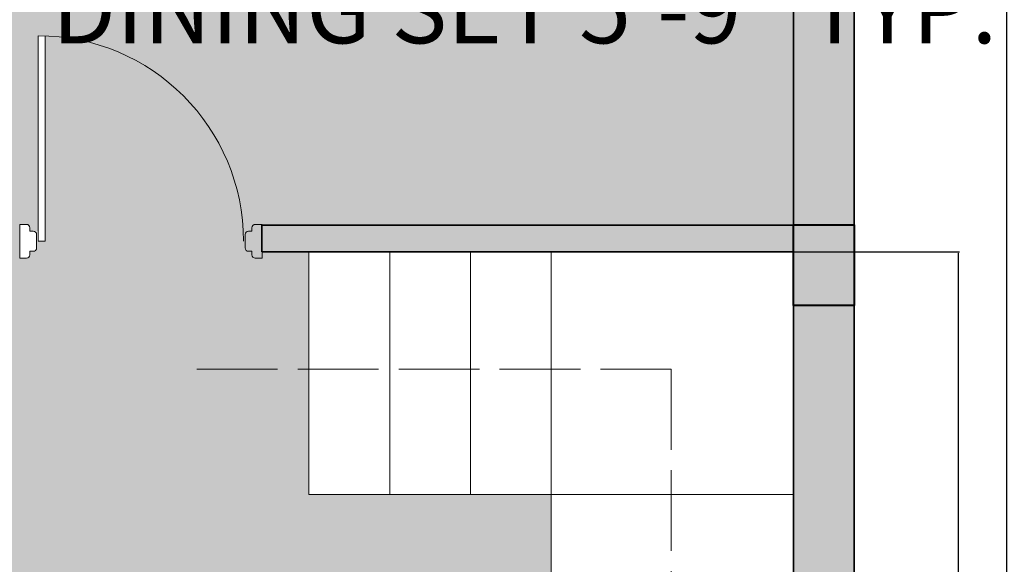
# Model space of a CAD drawing. Units: inches. Extents: x 1077 to 2505, y 1892 to 2728.
# Tile 9 of 26: x 1433 to 1579, y 2257 to 2338. Entities that reach past the tile are written whole.
import ezdxf

# ---------------------------------------------------------------- set-up
doc = ezdxf.new("R2010")
doc.units = ezdxf.units.IN
doc.linetypes.add('ACAD_ISO02W100', pattern=[15, 12, -3])
doc.layers.get('Defpoints').update_dxf_attribs({"color": 220, "linetype": 'ACAD_ISO02W100'})
for name, color, linetype, lineweight in [('00 FURNITURE', 15, 'Continuous', 15), ('A-ANNO-DIMS', 2, 'Continuous', 18), ('A-ANNO-STRS', 220, 'ACAD_ISO02W100', 13), ('A-COLS', 7, 'Continuous', 40), ('A-DOOR', 4, 'Continuous', 18), ('A-FLOR-FIXT', 8, 'Continuous', 13), ('A-FLOR-STRS', 7, 'Continuous', 18), ('A-WALL-PATT', 7, 'Continuous', 9), ('A_TEXT_SMALL', 18, 'Continuous', 13), ('WALL', 7, 'Continuous', 35)]:
    doc.layers.add(name, color=color, linetype=linetype, lineweight=lineweight)
doc.layers.add('A-FLOR-PATT', color=254, linetype='Continuous', lineweight=9, true_color=0xd7ebd2)
doc.styles.get("Standard").update_dxf_attribs({"font": 'arial.ttf'})
doc.dimstyles.get("Standard").update_dxf_attribs({"dimtxt": 10.18, "dimasz": 0.18, "dimexe": 0.18, "dimexo": 0.0625, "dimgap": 0.09, "dimtad": 0, "dimtih": 1, "dimtoh": 1, "dimdec": 0, "dimzin": 0, "dimdsep": 46, "dimlunit": 3, "dimtxsty": 'Standard', "dimcen": 0.09, "dimadec": 0, "dimazin": 0, "dimtfac": 1, "dimtdec": 0, "dimtofl": 0, "dimtmove": 0, "dimatfit": 3, "dimfxl": 1, "dimtolj": 1, "dimtzin": 0, "dimarcsym": 0})

# ---------------------------------------------------------------- blocks, each defined once
blk = doc.blocks.new('DDD')
at = {"layer": '00 FURNITURE'}
for p, q in [((-12579.77, -15859.53), (-12579.77, -15829.05)), ((-12578.77, -15859.53), (-12578.77, -15829.03)), ((-12612.02, -15857.03), (-12612.02, -15862.03)), ((-12611.02, -15857.03), (-12612.02, -15857.03)), ((-12610.52, -15858.03), (-12610.52, -15857.53)), ((-12577.52, -15858.03), (-12577.52, -15857.53)), ((-12577.02, -15857.03), (-12576.02, -15857.03)), ((-12576.02, -15857.03), (-12576.02, -15862.03)), ((-12578.77, -15859.53), (-12579.77, -15859.53)), ((-12612.02, -15862.03), (-12611.02, -15862.03)), ((-12610.52, -15861.53), (-12610.52, -15861.03)), ((-12577.52, -15861.53), (-12577.52, -15861.03)), ((-12576.02, -15862.03), (-12577.02, -15862.03))]:
    blk.add_line(p, q, dxfattribs=at)
for points in [[(-12610.52, -15861.03), (-12610.02, -15861.03, 0.414214), (-12609.52, -15860.53), (-12609.52, -15858.53, 0.414214), (-12610.02, -15858.03), (-12610.52, -15858.03)], [(-12577.52, -15861.03), (-12578.02, -15861.03, -0.414214), (-12578.52, -15860.53), (-12578.52, -15858.53, -0.414214), (-12578.02, -15858.03), (-12577.52, -15858.03)]]:
    blk.add_lwpolyline(points, format="xyb", dxfattribs=at)
for centre, radius, start, end in [((-12578.77, -15859.53), 30.5, 90, 180), ((-12611.02, -15857.53), 0.5, 0, 90), ((-12577.02, -15857.53), 0.5, 90, 180), ((-12611.02, -15861.53), 0.5, 270, 0), ((-12577.02, -15861.53), 0.5, 180, 270)]:
    blk.add_arc(centre, radius, start, end, dxfattribs=at)
blk = doc.blocks.new('reh-flat-2')
at = {"layer": 'A_TEXT_SMALL'}
for p, q in [((486053827.2, -394630231.2), (486054182.4, -394629799.8)), ((486054182.4, -394629799.8), (486054596.6, -394630140.9)), ((486053979.5, -394630126.3), (486054157.1, -394629910.6)), ((486054228.6, -394629903.6), (486054483.5, -394630113.5)), ((486054596.6, -394630140.9), (486054241.4, -394630572.3)), ((486054241.3, -394630407.7), (486053986.4, -394630197.8)), ((486054490.4, -394630185), (486054312.8, -394630400.7)), ((486054241.4, -394630572.3), (486053827.2, -394630231.2))]:
    blk.add_line(p, q, dxfattribs=at)
for centre, radius in [((486054234.9, -394630155.7), 38.1), ((486054004.1, -394630296.2), 20.1), ((486054072.7, -394630352.7), 20.1), ((486054141.4, -394630409.3), 20.1)]:
    blk.add_circle(centre, radius, dxfattribs=at)
for centre, start, end in [((486054196.3, -394629942.9), 50.5305, 140.5305), ((486054018.7, -394630158.5), 140.5305, 230.5305), ((486054451.2, -394630152.8), 320.5305, 50.5305), ((486054273.6, -394630368.4), 230.5305, 320.5305)]:
    blk.add_arc(centre, 50.8, start, end, dxfattribs=at)
blk = doc.blocks.new('C1')
h = blk.add_hatch(color=256)
h.dxf.hatch_style = 1
h.paths.add_polyline_path([(1668.56, 2445.41), (1677.56, 2445.41), (1677.56, 2457.41), (1668.56, 2457.41)])
for p, q in [((1668.56, 2457.41), (1677.56, 2457.41)), ((1668.56, 2445.41), (1668.56, 2457.41)), ((1677.56, 2457.41), (1677.56, 2445.41)), ((1677.56, 2445.41), (1668.56, 2445.41))]:
    blk.add_line(p, q)
blk = doc.blocks.new('*D14')
at = {"layer": 'A-ANNO-DIMS', "color": 0, "lineweight": -2, "transparency": 16777216}
for p, q in [((1555.59, 2651.66), (1579.43, 2651.66)), ((1579.25, 2651.48), (1579.25, 2375.3)), ((1579.25, 2088.54), (1579.25, 2364.72)), ((1555.59, 2088.36), (1579.43, 2088.36))]:
    blk.add_line(p, q, dxfattribs=at)
at = {"layer": 'A-ANNO-DIMS', "color": 0, "transparency": 16777216}
for points in [[(1579.22, 2651.48), (1579.28, 2651.48), (1579.25, 2651.66)], [(1579.22, 2088.54), (1579.28, 2088.54), (1579.25, 2088.36)]]:
    blk.add_solid(points, dxfattribs=at)
at = {"layer": 'Defpoints', "color": 0, "transparency": 16777216}
for p in [(1555.53, 2651.66), (1555.53, 2088.36), (1579.25, 2088.36)]:
    blk.add_point(p, dxfattribs=at)
at = {"layer": 'A-ANNO-DIMS', "color": 0, "transparency": 16777216, "insert": (1579.25, 2370.01), "char_height": 10.18, "attachment_point": 5}
blk.add_mtext('\\A1;46\'-11"', dxfattribs=at)
blk = doc.blocks.new('STAIR-PLAN-RETURN')
for p, q in [((0, 163.08), (0, 127.08)), ((12, 163.08), (12, 127.08)), ((24, 163.08), (24, 127.08)), ((36, 163.08), (36, 0)), ((36, 163.08), (36, 127.08)), ((0, 127.08), (72, 127.08))]:
    blk.add_line(p, q)
blk = doc.blocks.new('STAIR-DIRECTION')
for p, q in [((0, 107.9), (70.51, 107.9)), ((70.51, 107.9), (70.51, 0)), ((70.51, 0.8), (65.28, 12.48)), ((65.28, 12.48), (70.51, 1.21)), ((70.51, 0), (75.75, 12.88)), ((75.75, 12.88), (70.51, 0.8))]:
    blk.add_line(p, q)
blk = doc.blocks.new('*D36')
at = {"layer": 'A-ANNO-DIMS', "color": 0, "lineweight": -2, "transparency": 16777216}
for p, q in [((1365.09, 2349.48), (1365.09, 2339.05)), ((1433.87, 2349.48), (1433.87, 2339.05)), ((1365.27, 2339.23), (1433.69, 2339.23)), ((1433.87, 2339.23), (1434.05, 2339.23))]:
    blk.add_line(p, q, dxfattribs=at)
at = {"layer": 'A-ANNO-DIMS', "color": 0, "transparency": 16777216}
for points in [[(1365.27, 2339.26), (1365.27, 2339.2), (1365.09, 2339.23)], [(1433.69, 2339.26), (1433.69, 2339.2), (1433.87, 2339.23)]]:
    blk.add_solid(points, dxfattribs=at)
at = {"layer": 'Defpoints', "color": 0, "transparency": 16777216}
for p in [(1365.09, 2349.54), (1433.87, 2349.54), (1433.87, 2339.23)]:
    blk.add_point(p, dxfattribs=at)
at = {"layer": 'A-ANNO-DIMS', "color": 0, "transparency": 16777216, "insert": (1507.58, 2339.23), "char_height": 10.18, "attachment_point": 5}
blk.add_mtext('\\A1;DINING SET 5\'-9" TYP.', dxfattribs=at)
blk = doc.blocks.new('*D44')
at = {"layer": 'A-ANNO-DIMS', "color": 0, "lineweight": -2, "transparency": 16777216}
for p, q in [((1547.59, 2303.16), (1572.17, 2303.16)), ((1571.99, 2302.98), (1571.99, 2226.98)), ((1571.99, 2140.26), (1571.99, 2216.26)), ((1547.59, 2140.08), (1572.17, 2140.08))]:
    blk.add_line(p, q, dxfattribs=at)
at = {"layer": 'A-ANNO-DIMS', "color": 0, "transparency": 16777216}
for points in [[(1571.96, 2302.98), (1572.02, 2302.98), (1571.99, 2303.16)], [(1571.96, 2140.26), (1572.02, 2140.26), (1571.99, 2140.08)]]:
    blk.add_solid(points, dxfattribs=at)
at = {"layer": 'Defpoints', "color": 0, "transparency": 16777216}
for p in [(1547.53, 2303.16), (1571.99, 2303.16), (1547.53, 2140.08)]:
    blk.add_point(p, dxfattribs=at)
at = {"layer": 'A-ANNO-DIMS', "color": 0, "transparency": 16777216, "insert": (1571.99, 2221.62), "char_height": 10.18, "attachment_point": 5}
blk.add_mtext('\\A1;RETURN STAIR 13\'-7" TYP.', dxfattribs=at)

msp = doc.modelspace()

# ---------------------------------------------------------------- hatches: boundary and pattern name
at = {"layer": 'A-FLOR-PATT', "transparency": 33554559}
h = msp.add_hatch(color=256, dxfattribs=at)
h.dxf.hatch_style = 1
h.paths.add_polyline_path([(1395.53, 2577.16), (1374.83, 2577.16), (1350.83, 2577.19), (1350.83, 2577.16), (1329.53, 2577.16), (1329.53, 2480.16), (1329.53, 2469.16), (1325.53, 2469.16), (1325.53, 2515.13), (1307.53, 2515.13), (1307.53, 2577.16), (1269.31, 2577.16), (1221.31, 2577.15), (1221.31, 2577.16), (1187.53, 2577.16), (1187.53, 2433.16), (1289.53, 2433.16), (1289.53, 2429.16), (1263.53, 2429.16), (1187.53, 2429.16), (1187.53, 2395.02), (1187.53, 2395.02), (1187.53, 2371.02), (1187.53, 2371.02), (1187.53, 2307.16), (1259.53, 2307.16), (1259.53, 2399.16), (1263.53, 2399.16), (1263.53, 2307.16), (1289.53, 2307.16), (1289.53, 2306.23), (1325.53, 2306.23), (1325.53, 2307.16), (1329.53, 2307.16), (1329.53, 2306.23), (1365.53, 2306.23), (1365.53, 2307.16), (1432.53, 2307.16), (1432.53, 2088.16), (1547.53, 2088.16), (1547.53, 2140.08), (1511.53, 2140.08), (1511.53, 2267.16), (1475.53, 2267.16), (1475.53, 2303.16), (1468.53, 2303.16), (1468.53, 2307.16), (1547.53, 2307.16), (1547.53, 2348.22), (1547.53, 2396.22), (1547.53, 2429.16), (1435.53, 2429.16), (1435.53, 2433.16), (1476.35, 2433.16), (1476.35, 2451.18), (1547.53, 2451.18), (1547.53, 2577.16), (1499.53, 2577.16), (1499.53, 2586.16), (1547.53, 2586.16), (1547.53, 2642.16), (1518.18, 2642.16), (1518.18, 2642.05), (1494.15, 2642.05), (1494.15, 2642.16), (1469.53, 2642.16), (1469.53, 2577.16), (1399.53, 2577.16), (1399.53, 2429.16), (1325.53, 2429.16), (1325.53, 2433.16), (1329.53, 2433.16), (1395.53, 2433.16), (1395.53, 2480.16), (1359.53, 2480.16), (1359.53, 2484.16), (1395.53, 2484.16)])
h.paths.add_polyline_path([(1357.65, 2482.07), (1355.65, 2482.07), (1355.65, 2481.07, 0.414214), (1356.65, 2480.07), (1344.65, 2480.07), (1344.65, 2477.06), (1343.27, 2477.06), (1343.27, 2480.07), (1330.65, 2480.07, -0.414214), (1329.65, 2481.07), (1329.65, 2484.07), (1331.65, 2484.07), (1331.65, 2510.07, -0.446908)], flags=16)
h.paths.add_polyline_path([(1305.09, 2559.18), (1288.89, 2559.18), (1288.89, 2575.38), (1305.09, 2575.38)], flags=16)
h.paths.add_polyline_path([(1304.19, 2560.08), (1289.79, 2560.08), (1289.79, 2574.48), (1304.19, 2574.48)], flags=0)
h.paths.add_polyline_path([(1287.99, 2500.68, -0.414214), (1287.09, 2499.78), (1265.14, 2499.78), (1224.09, 2499.78, -0.414214), (1223.19, 2500.68), (1223.19, 2557.16), (1223.19, 2571.74), (1223.19, 2575.38), (1287.99, 2575.38), (1287.99, 2571.74), (1287.09, 2571.74, -0.414214), (1287.99, 2570.84)], flags=16)
h.paths.add_polyline_path([(1292.98, 2569.05, -1), (1300.92, 2569.05, -1)], flags=0)
h.paths.add_polyline_path([(1293.32, 2569.05, -1), (1300.58, 2569.05, -1)], flags=0)
h.paths.add_polyline_path([(1322.8, 2462.21), (1322.8, 2431.71), (1323.05, 2430.71), (1323.05, 2431.71), (1321.8, 2431.71), (1321.8, 2462.19, 0.404641), (1292.3, 2431.71), (1292.05, 2430.71, -0.414214), (1291.55, 2430.21), (1291.05, 2430.21), (1291.05, 2429.71, -0.414214), (1290.55, 2429.21), (1289.55, 2429.21), (1289.55, 2434.21), (1290.55, 2434.21, -0.414214), (1291.05, 2433.71), (1291.05, 2433.21), (1291.55, 2433.21, -0.414214), (1292.05, 2432.71), (1292.3, 2431.71, -0.414214)], flags=16)
h.paths.add_polyline_path([(1287.82, 2548.28, 0.292232), (1279.17, 2536.8, 0.052719), (1223.93, 2548.28), (1223.28, 2548.28), (1223.28, 2557.16), (1223.93, 2557.16), (1245.42, 2557.16, -0.117785), (1245.77, 2557.93, -0.059418), (1254.87, 2567.02, -0.379859), (1257.28, 2566.88, -0.02509), (1261.41, 2563.32, -0.025935), (1265.65, 2567.02, -0.379859), (1268.06, 2566.88, -0.061767), (1277.52, 2557.43, -0.069393), (1277.82, 2557.16), (1287.82, 2557.16)], flags=0)
h.paths.add_polyline_path([(1263.47, 2548.28), (1260.56, 2548.28, -0.015371), (1258.01, 2546.13, -0.429576), (1255.37, 2546.06, -0.016036), (1252.69, 2548.28), (1223.28, 2548.28), (1223.28, 2554.42), (1246.78, 2554.42, 0.055344), (1255.37, 2546.06, 0.331768), (1257.52, 2545.74, 0.027343), (1262, 2549.64, 0.00919)], flags=0)
h.paths.add_polyline_path([(1295.56, 2568.34), (1296.87, 2569.09), (1296.87, 2570.6, 0.399698), (1295.39, 2569.05, 0.119004)], flags=0)
h.paths.add_polyline_path([(1295.21, 2569.05, -1), (1298.68, 2569.05, -1)], flags=0)
h.paths.add_polyline_path([(1296.95, 2568.96), (1297.03, 2569), (1297.03, 2569.09), (1296.99, 2569.11), (1296.91, 2568.98)], flags=0)
h.paths.add_polyline_path([(1402.28, 2462.19, -0.414214), (1432.78, 2431.69), (1433.03, 2432.69), (1432.78, 2431.69, 0.404641), (1403.28, 2462.17), (1403.28, 2431.69), (1402.03, 2431.69), (1402.03, 2430.69, -0.414214), (1401.53, 2430.19), (1401.03, 2430.19), (1401.03, 2429.69, -0.414214), (1400.53, 2429.19), (1399.53, 2429.19), (1399.53, 2434.19), (1400.53, 2434.19, -0.414214), (1401.03, 2433.69), (1401.03, 2433.19), (1401.53, 2433.19, -0.414214), (1402.03, 2432.69)], flags=16)
h.paths.add_polyline_path([(1470.16, 2535.21, -0.414214), (1471.06, 2536.11), (1527.54, 2536.11), (1542.12, 2536.11), (1545.76, 2536.11), (1545.76, 2471.31), (1542.12, 2471.31), (1542.12, 2472.21, -0.414214), (1541.22, 2471.31), (1471.06, 2471.31, -0.414214), (1470.16, 2472.21), (1470.16, 2494.16)], flags=16)
h.paths.add_polyline_path([(1483.07, 2536.11, 0.253465), (1480.11, 2526.15, 0.2538), (1470.15, 2523.19)], flags=16)
h.paths.add_polyline_path([(1223.19, 2512.69, 0.253465), (1233.14, 2509.74, 0.2538), (1236.1, 2499.77)], flags=16)
h.paths.add_polyline_path([(1469.77, 2578.72), (1469.77, 2581.72), (1471.77, 2581.72), (1471.77, 2607.72, -0.01951), (1473.77, 2607.68), (1473.77, 2579.72), (1473.77, 2578.72, -0.414214), (1472.77, 2577.72), (1470.77, 2577.72, -0.414214)], flags=16)
h.paths.add_polyline_path([(1382.46, 2398.13), (1395.04, 2398.13), (1395.04, 2399.74), (1382.46, 2399.74)], flags=16)
h.paths.add_polyline_path([(1379.94, 2397.18), (1379.94, 2389.82), (1380.5, 2389.82), (1380.5, 2396.05, -0.41429), (1381.06, 2396.61), (1396.47, 2396.61, -0.414213), (1397.03, 2396.05), (1397.03, 2389.82), (1397.59, 2389.82), (1397.59, 2397.18)], flags=16)
h.paths.add_polyline_path([(1263.37, 2428.14), (1263.37, 2426.14, -0.414214), (1262.37, 2425.14), (1261.37, 2425.14), (1233.41, 2425.14, 0.400854), (1259.37, 2401.04), (1259.37, 2401.14), (1261.37, 2401.14, -0.446908), (1233.37, 2427.14), (1259.37, 2427.14), (1259.37, 2429.14), (1262.37, 2429.14, -0.414214)], flags=16)
h.paths.add_polyline_path([(1404.79, 2398.13), (1417.37, 2398.13), (1417.37, 2399.74), (1404.79, 2399.74)], flags=16)
h.paths.add_polyline_path([(1402.27, 2397.18), (1404.79, 2398.13), (1417.37, 2398.13), (1419.92, 2397.18)], flags=16)
h.paths.add_polyline_path([(1432.26, 2383.16), (1432.26, 2370.59), (1433.87, 2370.59), (1433.87, 2383.16)], flags=16)
h.paths.add_polyline_path([(1431.3, 2385.69), (1423.84, 2385.69), (1423.84, 2385.13), (1430.18, 2385.13, -0.41429), (1430.74, 2384.57), (1430.74, 2369.16, -0.414237), (1430.18, 2368.6), (1423.84, 2368.6), (1423.84, 2368.03), (1431.3, 2368.03)], flags=16)
h.paths.add_polyline_path([(1417.37, 2351.16), (1417.37, 2349.54), (1418.9, 2349.54, 0.414236), (1419.92, 2350.56), (1419.92, 2352.11)], flags=16)
h.paths.add_polyline_path([(1395.04, 2351.16), (1395.04, 2349.54), (1396.58, 2349.54, 0.414235), (1397.59, 2350.56), (1397.59, 2352.11)], flags=16)
h.paths.add_polyline_path([(1366.7, 2370.05), (1365.09, 2370.05), (1365.09, 2368.52, 0.414235), (1366.11, 2367.5), (1367.66, 2367.5)], flags=16)
h.paths.add_polyline_path([(1419.36, 2359.47), (1419.36, 2353.24, -0.41419), (1418.8, 2352.68), (1403.39, 2352.68, -0.414137), (1402.83, 2353.24), (1402.83, 2359.47), (1397.03, 2359.47), (1397.03, 2353.24, -0.414189), (1396.47, 2352.68), (1381.06, 2352.68, -0.414137), (1380.5, 2353.24), (1380.5, 2359.47)], flags=16)
h.paths.add_polyline_path([(1222.29, 2559.18), (1206.09, 2559.18), (1206.09, 2575.38), (1222.29, 2575.38)], flags=16)
h.paths.add_polyline_path([(1221.39, 2560.08), (1206.99, 2560.08), (1206.99, 2574.48), (1221.39, 2574.48)], flags=0)
h.paths.add_polyline_path([(1482, 2577.72), (1482, 2580.73), (1483.38, 2580.73), (1483.38, 2577.72), (1484.77, 2577.72), (1484.77, 2574.72), (1483.38, 2574.72), (1483.38, 2577.72)], flags=16)
h.paths.add_polyline_path([(1266.37, 2415.53), (1266.37, 2414.14), (1263.37, 2414.14), (1263.37, 2415.53), (1260.36, 2415.53), (1260.36, 2416.91), (1263.37, 2416.91), (1263.37, 2415.53)], flags=16)
h.paths.add_polyline_path([(1210.26, 2569.05, -1), (1218.19, 2569.05, -1)], flags=0)
h.paths.add_polyline_path([(1210.6, 2569.05, -1), (1217.85, 2569.05, -1)], flags=0)
h.paths.add_polyline_path([(1212.84, 2568.34), (1214.15, 2569.09), (1214.15, 2570.6, 0.399698), (1212.67, 2569.05, 0.119004)], flags=0)
h.paths.add_polyline_path([(1212.49, 2569.05, -1), (1215.96, 2569.05, -1)], flags=0)
h.paths.add_polyline_path([(1214.23, 2568.96), (1214.3, 2568.91), (1214.3, 2569)], flags=0)
h.paths.add_polyline_path([(1507.18, 2480.12, 0.052719), (1518.66, 2535.36), (1518.66, 2536.01), (1527.54, 2536.01), (1527.54, 2535.36), (1527.54, 2513.88, -0.117785), (1528.31, 2513.53, -0.059418), (1537.4, 2504.43, -0.379859), (1537.26, 2502.01, -0.02509), (1533.7, 2497.89, -0.025935), (1537.4, 2493.64, -0.379859), (1537.26, 2491.23, -0.061767), (1527.8, 2481.77, -0.069393), (1527.54, 2481.47), (1527.54, 2471.47), (1518.66, 2471.47, 0.292232)], flags=0)
h.paths.add_polyline_path([(1516.43, 2503.92, -0.016036), (1518.66, 2506.6), (1518.66, 2536.01), (1524.8, 2536.01), (1524.8, 2512.51, 0.055344), (1516.43, 2503.92, 0.331768), (1516.12, 2501.77, 0.027343), (1520.01, 2497.29, 0.00919), (1518.66, 2495.82), (1518.66, 2498.73, -0.015371), (1516.5, 2501.28, -0.429576)], flags=0)
h.paths.add_polyline_path([(1499.63, 2625.5, -0.171636), (1502.82, 2631.01), (1502.82, 2633.37), (1498.68, 2633.37, -0.414214), (1497.7, 2634.36), (1497.7, 2640.66, -0.414214), (1498.68, 2641.64), (1514.82, 2641.64, -0.414214), (1515.81, 2640.66), (1515.81, 2634.36, -0.414214), (1514.82, 2633.37), (1510.69, 2633.37), (1510.69, 2631.01, -0.171636), (1513.88, 2625.5, -0.258205), (1509.31, 2614.47), (1504.19, 2614.47, -0.258205)], flags=16)
h.paths.add_polyline_path([(1501.2, 2625.5, -0.171636), (1504.39, 2631.01), (1509.12, 2631.01, -0.171636), (1512.3, 2625.5, -0.210384), (1509.35, 2616.02), (1504.16, 2616.02, -0.210384)], flags=0)
h.paths.add_polyline_path([(1529.56, 2537.01), (1529.56, 2553.21), (1545.76, 2553.21), (1545.76, 2537.01)], flags=16)
h.paths.add_polyline_path([(1530.46, 2537.91), (1530.46, 2552.31), (1544.86, 2552.31), (1544.86, 2537.91)], flags=0)
h.paths.add_polyline_path([(1535.45, 2545.07, -1), (1543.39, 2545.07, -1)], flags=0)
h.paths.add_polyline_path([(1535.8, 2545.07, -1), (1543.05, 2545.07, -1)], flags=0)
h.paths.add_polyline_path([(1529.56, 2470.41), (1545.76, 2470.41), (1545.76, 2454.21), (1529.56, 2454.21)], flags=16)
h.paths.add_polyline_path([(1541.16, 2544.99), (1540.98, 2544.99, -0.544606), (1538.71, 2543.68), (1538.62, 2543.53, 0.547962)], flags=0)
h.paths.add_polyline_path([(1530.46, 2469.51), (1544.86, 2469.51), (1544.86, 2455.11), (1530.46, 2455.11)], flags=0)
h.paths.add_polyline_path([(1539.47, 2545.14), (1539.42, 2545.22), (1539.38, 2545.14)], flags=0)
h.paths.add_polyline_path([(1543.39, 2462.34, -1), (1535.45, 2462.34, -1)], flags=0)
h.paths.add_polyline_path([(1543.05, 2462.34, -1), (1535.8, 2462.34, -1)], flags=0)
h.paths.add_polyline_path([(1541.16, 2462.27), (1540.98, 2462.27, -0.544606), (1538.71, 2460.96), (1538.62, 2460.8, 0.547962)], flags=0)
h.paths.add_polyline_path([(1539.47, 2462.42), (1539.42, 2462.5), (1539.38, 2462.42)], flags=0)
h.paths.add_polyline_path([(1435.32, 2335.25, -0.414214), (1465.82, 2304.75), (1466.07, 2305.75), (1465.82, 2304.75, 0.404641), (1436.32, 2335.23), (1436.32, 2304.75), (1435.07, 2304.75), (1435.07, 2303.75, -0.414214), (1434.57, 2303.25), (1434.07, 2303.25), (1434.07, 2302.75, -0.414214), (1433.57, 2302.25), (1432.57, 2302.25), (1432.57, 2307.25), (1433.57, 2307.25, -0.414214), (1434.07, 2306.75), (1434.07, 2306.25), (1434.57, 2306.25, -0.414214), (1435.07, 2305.75)], flags=16)
h.paths.add_polyline_path([(1532.13, 2635.71), (1535.43, 2635.71), (1535.43, 2635.89), (1532.13, 2635.89)], flags=16)
edge = h.paths.add_edge_path(flags=16)
edge.add_arc((1535.98, 2632.67), 0.183, 270, 360)
edge.add_line((1536.17, 2632.67), (1536.17, 2639.82))
edge.add_line((1536.17, 2639.82), (1538.29, 2639.82))
edge.add_line((1538.29, 2639.82), (1538.29, 2641.82))
edge.add_line((1538.29, 2641.82), (1533.25, 2641.82))
edge.add_line((1533.25, 2641.82), (1533.25, 2639.82))
edge.add_line((1533.25, 2639.82), (1534.87, 2639.82))
edge.add_line((1534.87, 2639.82), (1534.87, 2639))
edge.add_line((1534.87, 2639), (1533.7, 2639))
edge.add_line((1533.7, 2639), (1533.7, 2639.82))
edge.add_line((1533.7, 2639.82), (1533.25, 2639.82))
edge.add_line((1533.25, 2639.82), (1533.25, 2641.82))
edge.add_line((1533.25, 2641.82), (1538.29, 2641.82))
edge.add_line((1538.29, 2641.82), (1538.29, 2641.34))
edge.add_line((1538.29, 2641.34), (1540.64, 2641.58))
edge.add_line((1540.64, 2641.58), (1540.64, 2641.82))
edge.add_line((1540.64, 2641.82), (1541.5, 2641.82))
edge.add_line((1541.5, 2641.82), (1541.5, 2641.25))
edge.add_line((1541.5, 2641.25), (1541.31, 2639.79))
edge.add_ellipse((1541.09, 2638.95), major_axis=(-1.08, 0), ratio=0.790849, start_angle=180, end_angle=255.2976, ccw=False)
edge.add_line((1542.17, 2638.95), (1542.17, 2638.38))
edge.add_ellipse((1541.09, 2638.38), major_axis=(-1.08, 0), ratio=0.790849, start_angle=0, end_angle=180, ccw=False)
edge.add_line((1540, 2638.38), (1540.01, 2638.87))
edge.add_ellipse((1541.09, 2638.95), major_axis=(-1.08, 0), ratio=0.790849, start_angle=284.7024, end_angle=364.0401, ccw=False)
edge.add_line((1540.78, 2639.75), (1540.78, 2641.25))
edge.add_line((1540.78, 2641.25), (1540.64, 2641.25))
edge.add_line((1540.64, 2641.25), (1538.29, 2641.01))
edge.add_line((1538.29, 2641.01), (1538.29, 2639.82))
edge.add_line((1538.29, 2639.82), (1536.17, 2639.82))
edge.add_line((1536.17, 2639.82), (1536.17, 2632.48))
edge.add_line((1536.17, 2632.48), (1535.98, 2632.48))
h.paths.add_polyline_path([(1496.32, 2250.34, -0.292371), (1498.9, 2247.83, -0.085148), (1501.21, 2208.85, -0.01331), (1500.27, 2098.5, -0.379287), (1497.22, 2095.28, -0.0502), (1441.54, 2095.28, -0.379287), (1438.5, 2098.5, -0.01331), (1437.56, 2208.85, -0.086132), (1439.96, 2248.26, -0.295116), (1442.59, 2250.78, -0.114238)], flags=16)
h.paths.add_polyline_path([(1495.16, 2205.84, -0.355389), (1496.7, 2202.1), (1492.94, 2189.65, -0.398275), (1489.12, 2187.47, 0.113332), (1449.64, 2187.47, -0.398275), (1445.82, 2189.65), (1442.06, 2202.1, -0.355394), (1443.6, 2205.84, -0.265725)], flags=0)
h.paths.add_polyline_path([(1440.37, 2195.72), (1445.94, 2181.67), (1445.94, 2160.63), (1440.84, 2157.26)], flags=0)
h.paths.add_polyline_path([(1498.46, 2195.72), (1497.99, 2157.26), (1492.88, 2160.63), (1492.88, 2181.67)], flags=0)
h.paths.add_polyline_path([(1445.94, 2158.37), (1445.94, 2137.12), (1441.12, 2122.56), (1440.87, 2155.03)], flags=0)
h.paths.add_polyline_path([(1492.88, 2158.37), (1497.96, 2155.03), (1497.71, 2122.56), (1492.88, 2137.12)], flags=0)
h.paths.add_polyline_path([(1489.88, 2130.4), (1494.39, 2107.67, -0.090102), (1444.44, 2107.65), (1448.95, 2130.39, 0.036636)], flags=0)
h.paths.add_polyline_path([(1447.54, 2159.34), (1497.44, 2159.34), (1497.44, 2177.89), (1447.54, 2177.89)], flags=8)
h.paths.add_polyline_path([(1196.44, 2354.84), (1246.65, 2354.84), (1246.65, 2388.43), (1196.44, 2388.43)], flags=24)
h.paths.add_polyline_path([(1296.09, 2360.25), (1353.81, 2360.25), (1353.81, 2393.84), (1296.09, 2393.84)], flags=24)
h.paths.add_polyline_path([(1400.72, 2471.85), (1470.63, 2471.85), (1470.63, 2505.44), (1400.72, 2505.44)], flags=24)
h.paths.add_polyline_path([(1324.78, 2448.48), (1394.95, 2448.48), (1394.95, 2467.02), (1324.78, 2467.02)], flags=24)
h.paths.add_polyline_path([(1335.08, 2531.43), (1389.67, 2531.43), (1389.67, 2565.02), (1335.08, 2565.02)], flags=24)
h.paths.add_polyline_path([(1225.76, 2460), (1295.67, 2460), (1295.67, 2493.58), (1225.76, 2493.58)], flags=24)
h = msp.add_hatch(color=256, dxfattribs=at)
h.dxf.hatch_style = 1
h.paths.add_polyline_path([(1547.53, 2348.22), (1547.53, 2396.22), (1547.53, 2425.11), (1547.53, 2425.11), (1547.53, 2429.16), (1435.53, 2429.16), (1434.03, 2429.21), (1434.03, 2430.19), (1433.03, 2430.19), (1432.78, 2431.69, 0.404641), (1403.28, 2462.17), (1403.28, 2431.69), (1402.03, 2431.69), (1402.03, 2430.19), (1401.03, 2430.19), (1401.03, 2429.19), (1399.53, 2429.19), (1399.53, 2429.19), (1399.53, 2429.16), (1334.67, 2429.16), (1334.67, 2423.95), (1325.67, 2423.95), (1325.67, 2429.16), (1325.53, 2429.16), (1324.05, 2429.24), (1324.05, 2430.21), (1323.05, 2430.21), (1323.05, 2431.71), (1321.8, 2431.71), (1321.8, 2462.19, 0.416544), (1292.05, 2430.73, -0.423614), (1291.55, 2430.21), (1291.05, 2430.21), (1291.05, 2429.21), (1289.55, 2429.21), (1289.53, 2429.21), (1289.53, 2429.16), (1263.37, 2429.16), (1263.37, 2415.53), (1266.37, 2415.53), (1266.37, 2414.14), (1263.37, 2414.14), (1263.37, 2399.16), (1263.53, 2399.16), (1263.53, 2307.16), (1289.53, 2307.16), (1289.53, 2306.23), (1323.26, 2306.23), (1323.26, 2307.21), (1332.26, 2307.21), (1365.53, 2306.23), (1365.53, 2307.16), (1432.53, 2307.16), (1432.57, 2307.16), (1432.57, 2307.25), (1434.07, 2307.25), (1434.07, 2306.25), (1435.32, 2306.25), (1435.32, 2335.25, -0.407346), (1466.07, 2305.73, -0.423614), (1466.57, 2306.25), (1467.07, 2306.25), (1467.07, 2307.25), (1468.57, 2307.25), (1547.53, 2307.16), (1547.53, 2307.2)])
h.paths.add_polyline_path([(1430.74, 2369.16), (1430.74, 2384.57, 0.41429), (1430.18, 2385.13), (1423.84, 2385.13), (1423.84, 2368.6), (1430.18, 2368.6, 0.414237)], flags=16)
h.paths.add_polyline_path([(1432.26, 2383.16), (1432.26, 2370.59), (1433.87, 2370.59), (1433.87, 2383.16)], flags=16)
h.paths.add_polyline_path([(1431.3, 2368.03), (1431.3, 2385.69), (1432.26, 2383.16), (1432.26, 2370.59)], flags=16)
h.paths.add_polyline_path([(1417.37, 2351.16), (1417.37, 2349.54), (1418.9, 2349.54, 0.414236), (1419.92, 2350.56), (1419.92, 2352.11)], flags=16)
h.paths.add_polyline_path([(1403.39, 2352.68), (1418.78, 2352.68, 0.42427), (1419.36, 2353.24), (1419.36, 2359.47), (1402.83, 2359.47), (1402.83, 2353.24, 0.414137)], flags=16)
h.paths.add_polyline_path([(1366.7, 2370.05), (1365.09, 2370.05), (1365.09, 2368.52, 0.414235), (1366.11, 2367.5), (1367.66, 2367.5)], flags=16)
h.paths.add_polyline_path([(1382.46, 2398.13), (1395.04, 2398.13), (1395.04, 2399.74), (1382.46, 2399.74)], flags=16)
h.paths.add_polyline_path([(1396.47, 2396.61), (1381.06, 2396.61, 0.41429), (1380.5, 2396.05), (1380.5, 2389.82), (1397.03, 2389.82), (1397.03, 2396.05, 0.414213)], flags=16)
h.paths.add_polyline_path([(1402.27, 2397.18), (1402.83, 2396.05, -0.414213), (1403.39, 2396.61)], flags=16)
h.paths.add_polyline_path([(1418.8, 2396.61), (1419.36, 2396.61), (1419.36, 2396.05, 0.414237)], flags=16)
h.paths.add_polyline_path([(1404.79, 2398.13), (1417.37, 2398.13), (1417.37, 2399.74), (1404.79, 2399.74)], flags=16)
h.paths.add_polyline_path([(1381.06, 2352.68, -0.414213), (1380.5, 2353.24), (1380.27, 2352.11)], flags=16)
h.paths.add_polyline_path([(1396.58, 2349.54), (1396.58, 2349.54), (1395.04, 2349.54), (1395.04, 2349.54), (1382.46, 2349.54), (1382.46, 2351.16), (1395.04, 2351.16), (1397.59, 2352.11), (1397.59, 2350.56, -0.414235)], flags=16)
h.paths.add_polyline_path([(1379.94, 2397.18), (1382.46, 2398.13), (1395.04, 2398.13), (1397.59, 2397.18)], flags=16)
h.paths.add_polyline_path([(1368.78, 2384.59, 0.414213), (1368.22, 2384.03), (1367.66, 2367.5), (1367.66, 2385.15)], flags=16)
h.paths.add_polyline_path([(1547.53, 2574.38), (1547.51, 2574.38), (1547.51, 2577.16), (1499.53, 2577.16), (1484.77, 2577.44), (1484.77, 2574.72), (1483.38, 2574.72), (1483.38, 2577.72), (1482, 2577.72), (1469.53, 2577.72), (1469.53, 2577.16), (1401.95, 2577.16), (1401.95, 2574.12), (1399.53, 2574.12), (1399.53, 2434.19), (1401.03, 2434.19), (1401.03, 2433.19), (1402.28, 2433.19), (1402.28, 2462.19, -0.407346), (1433.03, 2432.67, -0.423614), (1433.53, 2433.19), (1434.03, 2433.19), (1434.03, 2434.19), (1435.53, 2434.19), (1476.35, 2433.81), (1476.35, 2451.18), (1547.53, 2451.18)])
h.paths.add_polyline_path([(1470.16, 2535.21, -0.414214), (1471.06, 2536.11), (1527.54, 2536.11), (1542.12, 2536.11), (1545.76, 2536.11), (1545.76, 2471.31), (1542.12, 2471.31), (1542.12, 2472.21, -0.414214), (1541.22, 2471.31), (1471.06, 2471.31, -0.414214), (1470.16, 2472.21), (1470.16, 2494.16)], flags=16)
h.paths.add_polyline_path([(1483.07, 2536.11, 0.253465), (1480.11, 2526.15, 0.2538), (1470.15, 2523.19)], flags=16)
h.paths.add_polyline_path([(1525.55, 2481.52, -0.000893), (1524.8, 2482.24), (1524.8, 2471.47), (1527.54, 2471.47), (1527.54, 2472.12), (1527.54, 2481.47, -0.388819)], flags=0)
h.paths.add_polyline_path([(1518.66, 2536.01), (1527.54, 2536.01), (1527.54, 2535.36), (1527.54, 2513.88, -0.117785), (1528.31, 2513.53, -0.059418), (1537.4, 2504.43, -0.379859), (1537.26, 2502.01, -0.02509), (1533.7, 2497.89, 0.033431), (1528.3, 2502.74, 0.308459), (1526.25, 2502.88, 0.047827), (1518.66, 2495.82), (1518.66, 2498.73, -0.015371), (1516.5, 2501.28, -0.429576), (1516.43, 2503.92, -0.016036), (1518.66, 2506.6)], flags=0)
h.paths.add_polyline_path([(1529.56, 2537.01), (1529.56, 2553.21), (1545.76, 2553.21), (1545.76, 2537.01)], flags=16)
h.paths.add_polyline_path([(1530.46, 2537.91), (1530.46, 2552.31), (1544.86, 2552.31), (1544.86, 2537.91)], flags=0)
h.paths.add_polyline_path([(1535.8, 2545.07, -1), (1543.05, 2545.07, -1)], flags=0)
h.paths.add_polyline_path([(1541.16, 2544.99), (1540.98, 2544.99, -0.544606), (1538.71, 2543.68), (1538.62, 2543.53, 0.547962)], flags=0)
h.paths.add_polyline_path([(1539.47, 2545.14), (1539.42, 2545.22), (1539.38, 2545.14)], flags=0)
h.paths.add_polyline_path([(1529.56, 2470.41), (1545.76, 2470.41), (1545.76, 2454.21), (1529.56, 2454.21)], flags=16)
h.paths.add_polyline_path([(1530.46, 2469.51), (1544.86, 2469.51), (1544.86, 2455.11), (1530.46, 2455.11)], flags=0)
h.paths.add_polyline_path([(1535.8, 2462.34, -1), (1543.05, 2462.34, -1)], flags=0)
h.paths.add_polyline_path([(1541.16, 2462.27), (1540.98, 2462.27, -0.544606), (1538.71, 2460.96), (1538.62, 2460.8, 0.547962)], flags=0)
h.paths.add_polyline_path([(1539.47, 2462.42), (1539.42, 2462.5), (1539.38, 2462.42)], flags=0)
h.paths.add_polyline_path([(1395.53, 2574.12), (1392.95, 2574.12), (1392.95, 2577.16), (1374.83, 2577.16), (1350.83, 2577.19), (1350.83, 2577.16), (1332.07, 2577.16), (1332.07, 2574), (1329.53, 2574), (1329.53, 2484.07), (1331.65, 2484.07), (1331.65, 2510.07, -0.423677), (1357.76, 2484.07), (1359.53, 2484.07), (1359.53, 2484.16), (1395.53, 2484.16)], flags=17)
h.paths.add_polyline_path([(1395.53, 2480.16), (1359.06, 2480.16, 0.437533), (1359.53, 2481.55), (1359.53, 2484.16), (1395.53, 2484.16), (1395.53, 2574.12), (1392.95, 2574.12), (1392.95, 2577.16), (1374.83, 2577.16), (1350.83, 2577.19), (1350.83, 2577.16), (1332.07, 2577.16), (1332.07, 2574), (1329.53, 2574), (1329.53, 2484.07), (1329.65, 2484.07), (1329.65, 2481.07), (1329.53, 2480.16), (1329.53, 2469.16), (1325.53, 2469.16), (1325.53, 2515.13), (1307.53, 2515.13), (1307.53, 2577.16), (1269.31, 2577.16), (1221.31, 2577.15), (1221.31, 2577.16), (1187.61, 2577.16), (1187.61, 2574.03), (1187.53, 2433.16), (1289.55, 2433.16), (1289.55, 2434.21), (1291.05, 2434.21), (1291.05, 2433.21), (1292.05, 2433.21), (1292.3, 2431.71, -0.414214), (1322.8, 2462.21), (1323.05, 2432.71, -0.414214), (1323.55, 2433.21), (1324.05, 2433.21), (1324.05, 2434.21), (1325.67, 2434.21), (1325.67, 2435.95), (1334.67, 2435.95), (1334.67, 2433.16), (1395.53, 2433.16)])
h.paths.add_polyline_path([(1344.65, 2480.07), (1344.65, 2477.06), (1343.27, 2477.06), (1343.27, 2480.07), (1332.65, 2480.07, 0.414214), (1333.65, 2481.07), (1333.65, 2482.07), (1331.65, 2482.07), (1331.65, 2484.07), (1331.65, 2510.07, -0.446908), (1357.65, 2482.07), (1355.65, 2482.07), (1355.65, 2481.07, 0.414214), (1356.65, 2480.07)], flags=16)
h.paths.add_polyline_path([(1287.99, 2500.68, -0.414214), (1287.09, 2499.78), (1265.14, 2499.78), (1224.09, 2499.78, -0.414214), (1223.19, 2500.68), (1223.19, 2557.16), (1223.19, 2571.74), (1223.19, 2575.38), (1287.99, 2575.38), (1287.99, 2571.74), (1287.09, 2571.74, -0.414214), (1287.99, 2570.84)], flags=16)
h.paths.add_polyline_path([(1277.77, 2555.17, -0.000893), (1277.05, 2554.42), (1287.82, 2554.42), (1287.82, 2557.16), (1287.17, 2557.16), (1277.82, 2557.16, -0.388819)], flags=0)
h.paths.add_polyline_path([(1223.28, 2548.28), (1223.28, 2557.16), (1223.93, 2557.16), (1245.42, 2557.16, -0.117785), (1245.77, 2557.93, -0.059418), (1254.87, 2567.02, -0.379859), (1257.28, 2566.88, -0.02509), (1261.41, 2563.32, 0.033431), (1256.55, 2557.93, 0.308459), (1256.41, 2555.88, 0.047827), (1263.47, 2548.28), (1260.56, 2548.28, -0.015371), (1258.01, 2546.13, -0.429576), (1255.37, 2546.06, -0.016036), (1252.69, 2548.28)], flags=0)
h.paths.add_polyline_path([(1305.09, 2559.18), (1288.89, 2559.18), (1288.89, 2575.38), (1305.09, 2575.38)], flags=16)
h.paths.add_polyline_path([(1304.19, 2560.08), (1289.79, 2560.08), (1289.79, 2574.48), (1304.19, 2574.48)], flags=0)
h.paths.add_polyline_path([(1300.58, 2569.05, -1), (1293.32, 2569.05, -1)], flags=0)
h.paths.add_polyline_path([(1223.19, 2512.69, 0.253465), (1233.14, 2509.74, 0.2538), (1236.1, 2499.77)], flags=16)
h.paths.add_polyline_path([(1295.56, 2568.34), (1296.87, 2569.09), (1296.87, 2570.6, 0.399698), (1295.39, 2569.05, 0.119004)], flags=0)
h.paths.add_polyline_path([(1295.21, 2569.05, -1), (1298.68, 2569.05, -1)], flags=0)
h.paths.add_polyline_path([(1296.95, 2568.96), (1297.03, 2569), (1297.03, 2569.09), (1296.99, 2569.11), (1296.91, 2568.98)], flags=0)
h.paths.add_polyline_path([(1222.29, 2559.18), (1206.09, 2559.18), (1206.09, 2575.38), (1222.29, 2575.38)], flags=16)
h.paths.add_polyline_path([(1221.39, 2560.08), (1206.99, 2560.08), (1206.99, 2574.48), (1221.39, 2574.48)], flags=0)
h.paths.add_polyline_path([(1217.85, 2569.05, -1), (1210.6, 2569.05, -1)], flags=0)
h.paths.add_polyline_path([(1212.84, 2568.34), (1214.15, 2569.09), (1214.15, 2570.6, 0.399698), (1212.67, 2569.05, 0.119004)], flags=0)
h.paths.add_polyline_path([(1212.49, 2569.05, -1), (1215.96, 2569.05, -1)], flags=0)
h.paths.add_polyline_path([(1214.23, 2568.96), (1214.3, 2569), (1214.3, 2569.09), (1214.26, 2569.11), (1214.19, 2568.98)], flags=0)
h.paths.add_polyline_path([(1259.53, 2399.14), (1259.37, 2399.14), (1259.37, 2401.04, -0.423677), (1233.37, 2427.14), (1259.37, 2427.14), (1259.37, 2429.16), (1187.53, 2429.16), (1187.53, 2395.02), (1187.53, 2395.02), (1187.53, 2371.02), (1187.53, 2371.02), (1187.53, 2311.49), (1187.55, 2311.49), (1187.55, 2307.16), (1259.53, 2307.16)])
h.paths.add_polyline_path([(1323.26, 2295.21), (1323.26, 2304.23), (1289.53, 2304.23), (1289.53, 2303.16), (1187.55, 2303.16), (1187.55, 2299.49), (1178.53, 2299.49), (1178.53, 2267.66), (1178.53, 2219.66), (1182.03, 2219.66), (1182.03, 2267.67), (1184.03, 2267.67), (1184.03, 2219.66), (1187.53, 2219.66), (1187.53, 2153.16), (1228.13, 2153.16), (1276.13, 2153.16), (1276.13, 2153.16), (1324.54, 2153.16), (1324.54, 2154.67), (1325.54, 2154.67), (1325.54, 2155.92), (1296.54, 2155.92, -0.407346), (1326.06, 2186.67, -0.423614), (1325.54, 2187.17), (1325.54, 2187.67), (1324.54, 2187.67), (1324.54, 2189.17), (1325.43, 2295.21)])
h.paths.add_polyline_path([(1432.53, 2307.16), (1365.53, 2307.16), (1365.53, 2306.23), (1365.53, 2303.16), (1428.53, 2303.16), (1428.53, 2221.2), (1428.57, 2221.2), (1428.57, 2197.2), (1428.53, 2197.16), (1428.53, 2303.01), (1404.46, 2303.01), (1404.46, 2221.2), (1329.53, 2221.2), (1329.53, 2307.16), (1325.53, 2307.16), (1325.53, 2295.21), (1325.43, 2295.21), (1324.54, 2189.17), (1324.54, 2187.67), (1326.04, 2187.67, 1.016365), (1326.06, 2186.67, 0.407348), (1296.54, 2155.92), (1325.54, 2155.92), (1325.54, 2154.67), (1324.54, 2154.67), (1324.54, 2153.16), (1329.53, 2153.16), (1329.53, 2144.16), (1432.53, 2144.16)])
h.paths.add_polyline_path([(1361.95, 2194.26), (1361.95, 2193.16), (1329.53, 2193.16), (1329.53, 2189.16), (1329.54, 2188.17), (1329.54, 2189.16), (1329.53, 2189.16), (1329.53, 2193.16), (1361.95, 2193.16), (1361.95, 2196.26), (1409.95, 2196.26), (1409.95, 2194.26)], flags=16)
h.paths.add_polyline_path([(1377.02, 2200.5), (1345.91, 2200.5), (1345.91, 2218.4), (1347.87, 2218.4), (1347.87, 2219.18), (1374.75, 2219.18), (1374.75, 2218.4), (1377.02, 2218.4)], flags=16)
h.paths.add_polyline_path([(1367.07, 2210.7, -1), (1373.34, 2210.7, -1)], flags=0)
h.paths.add_polyline_path([(1349.92, 2210.7, -1), (1356.98, 2210.7, -1)], flags=0)
h.paths.add_polyline_path([(1405.95, 2256.57), (1405.95, 2277.6), (1427.86, 2277.6), (1427.86, 2256.57)], flags=16)
h.paths.add_polyline_path([(1412.92, 2258.68, -0.414201), (1410.93, 2260.67), (1410.93, 2273.62, -0.414239), (1412.92, 2275.61), (1423.88, 2275.61, -0.414227), (1425.87, 2273.62), (1425.87, 2260.67, -0.414214), (1423.88, 2258.68)], flags=0)
h.paths.add_polyline_path([(1407.61, 2263.66, -1), (1409.18, 2263.66, -1)], flags=0)
h.paths.add_polyline_path([(1407.61, 2267.14, -1), (1409.18, 2267.14, -1)], flags=0)
h.paths.add_polyline_path([(1416.91, 2267.15, -1), (1419.89, 2267.15, -1)], flags=0)
h.paths.add_polyline_path([(1407.61, 2270.63, -1), (1409.18, 2270.63, -1)], flags=0)
h.paths.add_polyline_path([(1475.53, 2303.16), (1468.57, 2303.16), (1468.57, 2302.25), (1467.07, 2302.25), (1467.07, 2303.25), (1466.07, 2303.25), (1465.82, 2304.75, 0.404641), (1436.32, 2335.23), (1436.32, 2304.75), (1435.07, 2304.75), (1435.07, 2303.25), (1434.07, 2303.25), (1434.07, 2302.25), (1432.53, 2302.25), (1432.53, 2144.16), (1432.53, 2088.16), (1547.52, 2088.16), (1547.52, 2100.19), (1547.52, 2140.08), (1511.53, 2140.08), (1511.53, 2267.16), (1475.53, 2267.16)])
h.paths.add_polyline_path([(1438.35, 2102.86, 0.033498), (1438.37, 2102.21, -0.000079)], flags=16)
h.paths.add_polyline_path([(1496.32, 2250.34, -0.292371), (1498.9, 2247.83, -0.085148), (1501.21, 2208.85, -0.012784), (1500.42, 2102.86, -0.033498), (1500.39, 2102.21, 0.012863), (1501.21, 2208.85, 0.077283), (1499.67, 2244.3, 0.265882), (1497.48, 2246.8, 0.14401), (1441.46, 2247.36, 0.270646), (1439.21, 2244.85, -0.007564), (1439.96, 2248.26, -0.295116), (1442.59, 2250.78, -0.114238)], flags=16)
h.paths.add_polyline_path([(1495.16, 2205.84, -0.355389), (1496.7, 2202.1), (1492.94, 2189.65, -0.398275), (1489.12, 2187.47, 0.113332), (1449.64, 2187.47, -0.398275), (1445.82, 2189.65), (1442.06, 2202.1, -0.355394), (1443.6, 2205.84, -0.265725)], flags=16)
h.paths.add_polyline_path([(1440.37, 2195.72), (1445.94, 2181.67), (1445.94, 2160.63), (1440.84, 2157.26)], flags=16)
h.paths.add_polyline_path([(1498.46, 2195.72), (1497.99, 2157.26), (1492.88, 2160.63), (1492.88, 2181.67)], flags=16)
h.paths.add_polyline_path([(1445.94, 2158.37), (1445.94, 2137.12), (1441.12, 2122.56), (1440.87, 2155.03)], flags=16)
h.paths.add_polyline_path([(1492.88, 2158.37), (1497.96, 2155.03), (1497.71, 2122.56), (1492.88, 2137.12)], flags=16)
h.paths.add_polyline_path([(1489.88, 2130.4), (1494.39, 2107.67, -0.090102), (1444.44, 2107.65), (1448.95, 2130.39, 0.036636)], flags=16)
h.paths.add_polyline_path([(1296.09, 2360.25), (1353.81, 2360.25), (1353.81, 2393.84), (1296.09, 2393.84)], flags=24)
h.paths.add_polyline_path([(1400.72, 2471.85), (1470.63, 2471.85), (1470.63, 2505.44), (1400.72, 2505.44)], flags=24)
h.paths.add_polyline_path([(1335.08, 2531.43), (1389.67, 2531.43), (1389.67, 2565.02), (1335.08, 2565.02)], flags=24)
h.paths.add_polyline_path([(1324.78, 2448.48), (1394.95, 2448.48), (1394.95, 2467.02), (1324.78, 2467.02)], flags=24)
h.paths.add_polyline_path([(1225.76, 2460), (1295.67, 2460), (1295.67, 2493.58), (1225.76, 2493.58)], flags=24)
h.paths.add_polyline_path([(1196.44, 2354.84), (1246.65, 2354.84), (1246.65, 2388.43), (1196.44, 2388.43)], flags=24)
h.paths.add_polyline_path([(1447.54, 2159.34), (1497.44, 2159.34), (1497.44, 2177.89), (1447.54, 2177.89)], flags=24)
at = {"layer": 'A-WALL-PATT', "transparency": 33554585}
h = msp.add_hatch(color=256, dxfattribs=at)
h.dxf.hatch_style = 1
h.paths.add_polyline_path([(1187.53, 2424), (1178.53, 2424), (1178.53, 2395.02), (1187.53, 2395.02)])
h.paths.add_polyline_path([(1187.53, 2371.02), (1178.53, 2371.02), (1178.53, 2311.49), (1187.53, 2311.49)])
h.paths.add_polyline_path([(1228.13, 2153.16), (1187.53, 2153.16), (1187.53, 2219.66), (1178.53, 2219.66), (1178.53, 2100.18), (1187.53, 2100.18), (1187.53, 2144.16), (1228.13, 2144.16)])
h.paths.add_polyline_path([(1432.53, 2097.16), (1187.53, 2097.16), (1187.53, 2100.18), (1178.53, 2100.18), (1178.53, 2088.16), (1432.53, 2088.16)])
h.paths.add_polyline_path([(1556.53, 2348.22), (1547.53, 2348.22), (1547.53, 2348.22), (1547.53, 2307.16), (1468.53, 2307.16), (1468.53, 2303.16), (1547.53, 2303.16), (1547.53, 2088.16), (1556.53, 2088.16)])
h.paths.add_polyline_path([(1556.53, 2425.11), (1547.53, 2425.11), (1547.53, 2396.22), (1556.53, 2396.22)])
h.paths.add_polyline_path([(1547.53, 2433.16), (1435.53, 2433.16), (1435.53, 2429.16), (1547.53, 2429.16)])
h.paths.add_polyline_path([(1556.53, 2574.38), (1547.53, 2574.38), (1547.53, 2451.18), (1547.55, 2451.18), (1547.55, 2437.11), (1556.53, 2437.11)])
h.paths.add_polyline_path([(1556.53, 2639.11), (1547.53, 2639.11), (1547.53, 2586.38), (1556.53, 2586.38)])
h.paths.add_polyline_path([(1556.53, 2639.11), (1547.53, 2639.11), (1547.53, 2642.16), (1518.18, 2642.16), (1518.18, 2642.05), (1494.18, 2642.05), (1494.18, 2651.05), (1518.15, 2651.05), (1518.15, 2651.16), (1556.53, 2651.16)])
h.paths.add_polyline_path([(1494.15, 2651.16), (1469.6, 2651.16), (1469.6, 2642.16), (1494.15, 2642.16)])
h.paths.add_polyline_path([(1221.31, 2577.16), (1187.61, 2577.16), (1187.61, 2574.03), (1178.61, 2574.03), (1178.61, 2586.16), (1221.31, 2586.16)])
h.paths.add_polyline_path([(1323.07, 2586.16), (1269.31, 2586.16), (1269.31, 2577.16), (1323.07, 2577.16)])
h.paths.add_polyline_path([(1374.84, 2586.19), (1374.84, 2577.19), (1350.84, 2577.19), (1350.83, 2577.19), (1350.83, 2577.16), (1332.07, 2577.16), (1332.07, 2574), (1323.07, 2574), (1323.07, 2586.16), (1350.83, 2586.16), (1350.84, 2586.16), (1350.84, 2586.19)])
h.paths.add_polyline_path([(1392.95, 2586.16), (1374.84, 2586.16), (1374.84, 2577.16), (1392.95, 2577.16)], flags=17)
h.paths.add_polyline_path([(1469.53, 2642.16), (1469.6, 2651.16), (1460.53, 2651.16), (1460.53, 2586.16), (1392.95, 2586.16), (1392.95, 2577.16), (1395.53, 2577.16), (1395.53, 2484.16), (1359.53, 2484.16), (1359.53, 2480.16), (1395.53, 2480.16), (1395.53, 2433.16), (1329.53, 2433.16), (1325.53, 2433.16), (1325.53, 2429.16), (1399.53, 2429.16), (1399.53, 2577.16), (1469.53, 2577.16)])
h.paths.add_polyline_path([(1187.53, 2574.03), (1178.53, 2574.03), (1178.53, 2436), (1187.53, 2436)])

# ---------------------------------------------------------------- linework, layer by layer
at = {"layer": 'WALL'}
for p, q in [((1547.53, 2348.22), (1547.53, 2307.16)), ((1556.53, 2348.22), (1556.53, 2088.16)), ((1468.53, 2307.16), (1547.53, 2307.16)), ((1468.53, 2303.16), (1468.53, 2307.16)), ((1468.53, 2303.16), (1547.53, 2303.16)), ((1547.53, 2303.16), (1547.53, 2088.16))]:
    msp.add_line(p, q, dxfattribs=at)

# ---------------------------------------------------------------- block references
at = {"layer": 'A-ANNO-STRS'}
msp.add_blockref('STAIR-DIRECTION', (1458.86, 2177.87), dxfattribs=at)
at = {"layer": 'A-COLS'}
msp.add_blockref('C1', (-121.03, -150.21), dxfattribs=at)
at = {"layer": 'A-DOOR', "xscale": -1}
msp.add_blockref('DDD', (-11143.46, 18164.28), dxfattribs=at)
at = {"layer": 'A-FLOR-FIXT', "xscale": 0.0391972730482577, "yscale": 0.0391972730482577, "zscale": 0.0391972730482577, "rotation": 309.4694759622496}
msp.add_blockref('reh-flat-2', (-168252.82, 24542481.88), dxfattribs=at)
at = {"layer": 'A-FLOR-STRS'}
msp.add_blockref('STAIR-PLAN-RETURN', (1475.53, 2140.08), dxfattribs=at)

# ---------------------------------------------------------------- dimensions: what is measured, and where the dimension line sits
at = {"layer": 'A-ANNO-DIMS'}
dim = msp.add_linear_dim(base=(1579.25, 2088.36), p1=(1555.53, 2651.66), p2=(1555.53, 2088.36), angle=90, dimstyle='Standard', override={"dimclrd": 0, "dimclre": 0, "dimclrt": 0}, dxfattribs=at)
dim.commit()
dim.dimension.update_dxf_attribs({"geometry": '*D14', "text_midpoint": (1579.25, 2370.01)})
dim = msp.add_linear_dim(base=(1433.87, 2339.23), p1=(1365.09, 2349.54), p2=(1433.87, 2349.54), text='DINING SET <> TYP.', dimstyle='Standard', override={"dimdec": 1, "dimlfac": 1, "dimrnd": 0, "dimzin": 1, "dimdsep": 46, "dimlunit": 4, "dimfrac": 2}, dxfattribs=at)
dim.commit()
dim.dimension.update_dxf_attribs({"geometry": '*D36', "text_midpoint": (1507.58, 2339.23)})
dim = msp.add_linear_dim(base=(1571.99, 2303.16), p1=(1547.53, 2140.08), p2=(1547.53, 2303.16), angle=90, text='RETURN STAIR <> TYP.', dimstyle='Standard', override={"dimdec": 1, "dimlfac": 1, "dimrnd": 0, "dimzin": 1, "dimdsep": 46, "dimlunit": 4, "dimfrac": 2}, dxfattribs=at)
dim.commit()
dim.dimension.update_dxf_attribs({"geometry": '*D44', "text_midpoint": (1571.99, 2221.62)})

doc.saveas('drawing.dxf')
